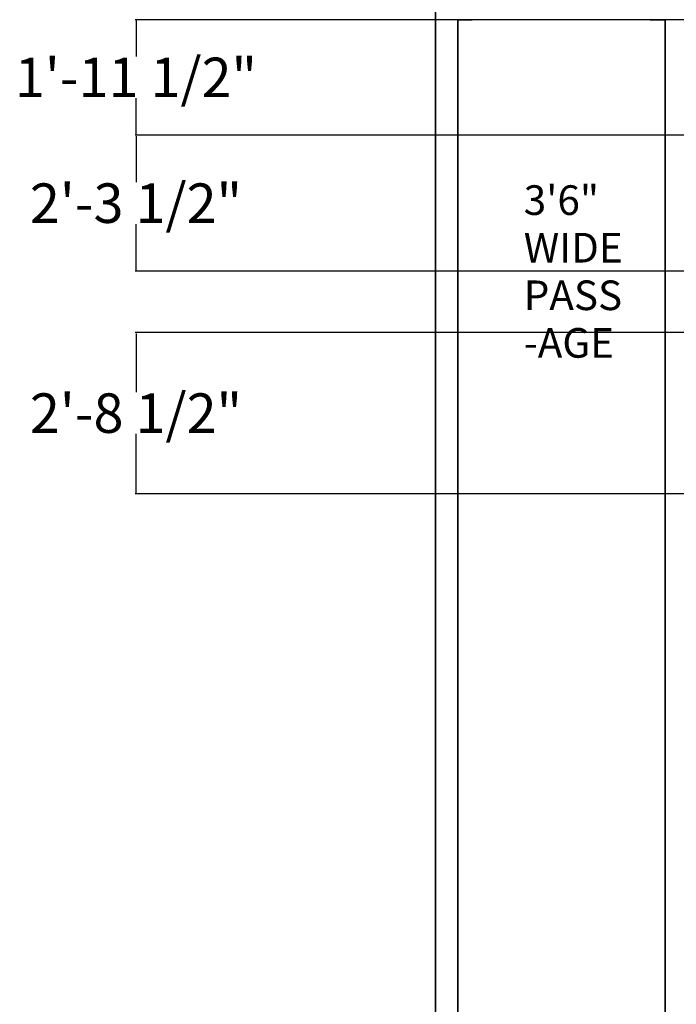
# Model space of a CAD drawing. Units: inches. Extents: x -438 to 102, y -60 to 1091.
# Tile 6 of 20: x -438 to -305, y 699 to 898. Entities that reach past the tile are written whole.
import ezdxf

# ---------------------------------------------------------------- set-up
doc = ezdxf.new("R2010")
doc.units = ezdxf.units.IN
doc.header["$MEASUREMENT"] = 0
for name, color, linetype, lineweight, true_color in [('A-ANNO-DIMS', 217, 'Continuous', 18, 0x93278f), ('A-WALL', 2, 'Continuous', 35, 0xf1eb1f), ('C-PROP', 2, 'Continuous', 35, 0xf1eb1f)]:
    doc.layers.add(name, color=color, linetype=linetype, lineweight=lineweight, true_color=true_color)
doc.layers.add('A-AREA-IDEN', color=4, linetype='Continuous', lineweight=18)
doc.styles.get("Standard").update_dxf_attribs({"font": 'arial.ttf'})
doc.dimstyles.get("Standard").update_dxf_attribs({"dimtxt": 8, "dimasz": 0.18, "dimexe": 0.18, "dimexo": 0.0625, "dimgap": 0.09, "dimtad": 0, "dimtih": 1, "dimtoh": 1, "dimdec": 4, "dimzin": 0, "dimdsep": 46, "dimlunit": 3, "dimtxsty": 'Standard', "dimcen": 0.09, "dimadec": 0, "dimazin": 0, "dimtfac": 1, "dimtdec": 4, "dimtofl": 0, "dimtmove": 0, "dimatfit": 3, "dimfxl": 1, "dimtolj": 1, "dimtzin": 0, "dimarcsym": 0})

# ---------------------------------------------------------------- blocks, each defined once
blk = doc.blocks.new('*D42')
at = {"layer": 'A-ANNO-DIMS', "color": 0, "lineweight": -2, "transparency": 16777216}
for p, q in [((-266, 834.64), (-414.94, 834.64)), ((-414.76, 834.46), (-414.76, 822.55)), ((-414.76, 802.18), (-414.76, 814.09)), ((-303.21, 802), (-414.94, 802))]:
    blk.add_line(p, q, dxfattribs=at)
at = {"layer": 'A-ANNO-DIMS', "color": 0, "transparency": 16777216}
for points in [[(-414.79, 834.46), (-414.73, 834.46), (-414.76, 834.64)], [(-414.79, 802.18), (-414.73, 802.18), (-414.76, 802)]]:
    blk.add_solid(points, dxfattribs=at)
at = {"layer": 'Defpoints', "color": 0, "transparency": 16777216}
for p in [(-414.76, 834.64), (-265.94, 834.64), (-303.15, 802)]:
    blk.add_point(p, dxfattribs=at)
at = {"layer": 'A-ANNO-DIMS', "color": 0, "transparency": 16777216, "insert": (-414.76, 818.32), "char_height": 8, "attachment_point": 5}
blk.add_mtext('\\A1;2\'-8 1/2"', dxfattribs=at)
blk = doc.blocks.new('*D52')
at = {"layer": 'A-ANNO-DIMS', "color": 0, "lineweight": -2, "transparency": 16777216}
for p, q in [((-291.6, 874.62), (-414.94, 874.62)), ((-414.76, 874.44), (-414.76, 865.07)), ((-414.76, 847.24), (-414.76, 856.61)), ((-291.6, 847.06), (-414.94, 847.06))]:
    blk.add_line(p, q, dxfattribs=at)
at = {"layer": 'A-ANNO-DIMS', "color": 0, "transparency": 16777216}
for points in [[(-414.79, 874.44), (-414.73, 874.44), (-414.76, 874.62)], [(-414.79, 847.24), (-414.73, 847.24), (-414.76, 847.06)]]:
    blk.add_solid(points, dxfattribs=at)
at = {"layer": 'Defpoints', "color": 0, "transparency": 16777216}
for p in [(-414.76, 874.62), (-291.54, 874.62), (-291.54, 847.06)]:
    blk.add_point(p, dxfattribs=at)
at = {"layer": 'A-ANNO-DIMS', "color": 0, "transparency": 16777216, "insert": (-414.76, 860.84), "char_height": 8, "attachment_point": 5}
blk.add_mtext('\\A1;2\'-3 1/2"', dxfattribs=at)
blk = doc.blocks.new('*D56')
at = {"layer": 'A-ANNO-DIMS', "color": 0, "lineweight": -2, "transparency": 16777216}
for p, q in [((-303.21, 898), (-414.94, 898)), ((-414.76, 897.82), (-414.76, 890.54)), ((-414.76, 874.8), (-414.76, 882.08)), ((-291.6, 874.62), (-414.94, 874.62))]:
    blk.add_line(p, q, dxfattribs=at)
at = {"layer": 'A-ANNO-DIMS', "color": 0, "transparency": 16777216}
for points in [[(-414.79, 897.82), (-414.73, 897.82), (-414.76, 898)], [(-414.79, 874.8), (-414.73, 874.8), (-414.76, 874.62)]]:
    blk.add_solid(points, dxfattribs=at)
at = {"layer": 'Defpoints', "color": 0, "transparency": 16777216}
for p in [(-414.76, 898), (-303.15, 898), (-291.54, 874.62)]:
    blk.add_point(p, dxfattribs=at)
at = {"layer": 'A-ANNO-DIMS', "color": 0, "transparency": 16777216, "insert": (-414.76, 886.31), "char_height": 8, "attachment_point": 5}
blk.add_mtext('\\A1;1\'-11 1/2"', dxfattribs=at)

msp = doc.modelspace()

# ---------------------------------------------------------------- linework, layer by layer
at = {"layer": 'A-WALL'}
for p, q in [((-346.7047, 897.99939), (-349.64649, 897.99939)), ((-307.64649, 897.99939), (-310.7047, 897.99939)), ((-307.64649, 897.99939), (-307.64649, 579.99939))]:
    msp.add_line(p, q, dxfattribs=at)
at = {"layer": 'C-PROP'}
for p, q in [((-354.14649, 1026.99939), (-354.14649, 3.99939)), ((-349.64649, 897.99939), (-349.64649, 8.49939))]:
    msp.add_line(p, q, dxfattribs=at)

# ---------------------------------------------------------------- texts
at = {"layer": 'A-AREA-IDEN'}
for s, p in [('3\'6"', (-336.27826, 858.45764)), ('WIDE', (-336.27826, 848.81916)), ('PASS', (-336.27826, 839.18069)), ('-AGE', (-336.27826, 829.54222))]:
    msp.add_text(s, height=6, dxfattribs=at).set_placement(p)

# ---------------------------------------------------------------- dimensions: what is measured, and where the dimension line sits
at = {"layer": 'A-ANNO-DIMS'}
for base, p1, p2, picture, middle in [((-414.76009, 897.99939), (-291.54025, 874.62295), (-303.14649, 897.99939), '*D56', (-414.76009, 886.31117)), ((-414.76009, 874.62295), (-291.54025, 847.06395), (-291.54025, 874.62295), '*D52', (-414.76009, 860.84345)), ((-414.76009, 834.64014), (-303.14649, 801.99939), (-265.93641, 834.64014), '*D42', (-414.76009, 818.31976))]:
    dim = msp.add_linear_dim(base=base, p1=p1, p2=p2, angle=90, dimstyle='Standard', override={"dimdec": 1, "dimlfac": 1, "dimrnd": 0, "dimzin": 1, "dimdsep": 46, "dimlunit": 4, "dimfrac": 2}, dxfattribs=at)
    dim.commit()
    dim.dimension.update_dxf_attribs({"geometry": picture, "text_midpoint": middle})

doc.saveas('drawing.dxf')
